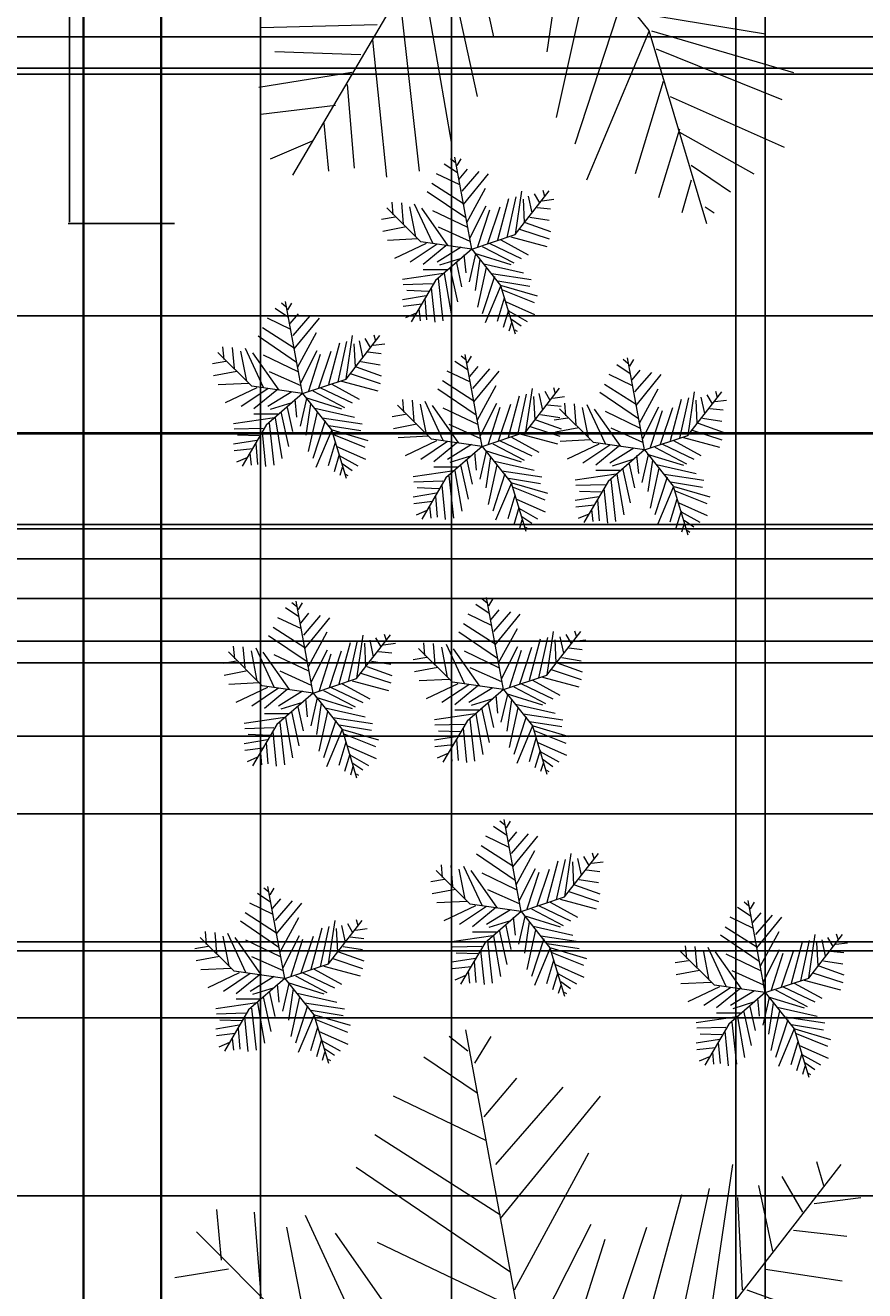
# Model space of a CAD drawing. Units: inches. Extents: x 818 to 1898, y 976 to 2364.
# Tile 6 of 96: x 986 to 1083, y 1446 to 1592. Entities that reach past the tile are written whole.
import ezdxf

# ---------------------------------------------------------------- set-up
doc = ezdxf.new("R2010")
doc.units = ezdxf.units.IN
doc.header["$LTSCALE"] = 5
doc.header["$MEASUREMENT"] = 0
for name, color, linetype, lineweight in [('A-ANNO-DIMS', 2, 'Continuous', 18), ('C-PROP', 7, 'Continuous', 35), ('L-PLNT-BEDS', 94, 'Continuous', 18)]:
    doc.layers.add(name, color=color, linetype=linetype, lineweight=lineweight)
doc.layers.add('L-PLNT', color=116, linetype='Continuous', lineweight=13, true_color=0x136734)
doc.styles.get("Standard").update_dxf_attribs({"font": 'arial.ttf'})
doc.dimstyles.get("Standard").update_dxf_attribs({"dimtxt": 0.18, "dimasz": 0.18, "dimexe": 0.18, "dimexo": 0.0625, "dimgap": 0.09, "dimtad": 0, "dimtih": 1, "dimtoh": 1, "dimdec": 4, "dimzin": 0, "dimdsep": 46, "dimtxsty": 'Standard', "dimcen": 0.09, "dimadec": 0, "dimazin": 0, "dimtfac": 1, "dimtdec": 4, "dimtofl": 0, "dimtmove": 0, "dimatfit": 3, "dimfxl": 1, "dimtolj": 1, "dimtzin": 0, "dimarcsym": 0})

# ---------------------------------------------------------------- blocks, each defined once
blk = doc.blocks.new('SHRUB-ACCENT')
for p, q in [((8.8, 18.63), (7.25, 19.67)), ((8.53, 19.84), (7.99, 20.28)), ((10.44, 9.82), (8.47, 20.47)), ((8.74, 19.5), (9.21, 20.28)), ((9.01, 17.93), (9.96, 19.06)), ((9.08, 17.24), (6.37, 18.54)), ((9.35, 16.54), (11.31, 18.8)), ((9.48, 14.98), (12.39, 18.54)), ((9.75, 13.42), (5.28, 16.46)), ((9.48, 15.07), (5.82, 17.41)), ((9.89, 12.9), (12.06, 16.89)), ((15.49, 11.5), (19.41, 16.55)), ((15.51, 11.51), (16.25, 16.54)), ((17.68, 16.2), (18.29, 15.16)), ((18.69, 16.63), (18.9, 15.94)), ((1.35, 13.77), (1.22, 15.24)), ((2.3, 15.16), (2.51, 12.72)), ((3.25, 14.72), (3.93, 11.25)), ((3.79, 15.07), (5.89, 10.55)), ((10.23, 11.07), (12.12, 14.81)), ((12.33, 10.47), (13.75, 14.72)), ((13.48, 10.9), (14.76, 15.68)), ((14.56, 11.16), (15.58, 15.85)), ((16.39, 15.59), (16.53, 12.9)), ((17, 15.94), (17.41, 14.03)), ((18.62, 15.42), (19.98, 15.59)), ((1.56, 13.51), (0, 13.25)), ((4.55, 10.66), (0.62, 14.58)), ((7.72, 10.21), (4.67, 14.55)), ((5.89, 14.29), (9.89, 12.38)), ((11.17, 10.12), (12.53, 14.37)), ((17.2, 13.51), (19.44, 13.16)), ((18.02, 14.63), (19.57, 14.46)), ((2.84, 12.38), (0.14, 11.86)), ((6.57, 12.38), (10.23, 10.73)), ((15.98, 12.12), (19.44, 10.99)), ((16.66, 12.9), (19.57, 11.86)), ((4.2, 10.99), (0.68, 10.81)), ((5.15, 10.47), (1.49, 8.73)), ((6.43, 10.38), (3.32, 8.3)), ((10.44, 9.82), (4.55, 10.66)), ((10.44, 9.82), (15.49, 11.5)), ((12.53, 10.47), (16.19, 8.73)), ((13.82, 10.9), (17, 9.16)), ((14.97, 11.25), (19.17, 10.12)), ((7.45, 10.21), (4.81, 8.04)), ((10.44, 9.82), (6.23, 6.17)), ((9.21, 10.03), (6.43, 8.3)), ((9.55, 9.16), (9.75, 7.08)), ((10.9, 9.25), (10.16, 6.04)), ((10.44, 9.82), (13.8, 5.61)), ((10.77, 9.34), (14.97, 8.04)), ((11.65, 10.12), (15.31, 8.21)), ((7.59, 7.43), (4.81, 7.43)), ((9.21, 8.73), (6.7, 7.95)), ((7.92, 7.69), (8.8, 3.69)), ((8.67, 8.21), (9.28, 5.43)), ((11.38, 8.64), (10.84, 5)), ((12.12, 7.69), (11.11, 3.09)), ((11.85, 8.12), (16.46, 7.08)), ((7.18, 6.99), (2.44, 6.3)), ((6.23, 6.17), (3.43, 1.4)), ((6.57, 6.39), (7.11, 1.52)), ((7.25, 6.99), (8.06, 2.31)), ((13.07, 6.65), (11.65, 2.31)), ((12.73, 6.99), (17.34, 6.3)), ((13.48, 6.13), (17.2, 5.52)), ((5.89, 5.78), (2.51, 5.69)), ((5.42, 4.91), (2.91, 5)), ((5.76, 5.34), (6.16, 1.35)), ((13.82, 5.6), (11.99, 1.26)), ((13.8, 5.61), (15.49, 0)), ((13.88, 5.6), (18.02, 4.39)), ((14.02, 5.08), (17.68, 3.61)), ((5.15, 4.39), (2.44, 3.95)), ((4.67, 3.43), (2.51, 3.17)), ((5.01, 4.04), (5.21, 1.61)), ((14.22, 4.13), (13.41, 1.44)), ((14.43, 3.69), (17.74, 2.22)), ((4, 2.39), (2.78, 1.87)), ((4.33, 2.91), (4.47, 1.52)), ((14.7, 2.74), (14.09, 0.74)), ((14.7, 2.65), (16.86, 1.44)), ((15.04, 1.7), (16.19, 0.92)), ((15.04, 1.26), (14.76, 0.31)), ((15.44, 0.48), (15.71, 0.31))]:
    blk.add_line(p, q)
blk = doc.blocks.new('PALM-BORDER')
for p, q in [((33.95, 78.95), (31.8, 80.68)), ((41.53, 39.05), (33.72, 81.45)), ((34.76, 77.57), (36.65, 80.68)), ((35.03, 74.11), (28.83, 78.26)), ((35.84, 71.35), (39.61, 75.84)), ((37.18, 65.82), (45, 74.8)), ((36.11, 68.59), (25.33, 73.77)), ((37.72, 59.6), (49.31, 73.77)), ((37.72, 59.95), (23.17, 69.28)), ((39.34, 51.31), (47.96, 67.2)), ((74.37, 66.17), (75.18, 63.4)), ((38.8, 53.39), (21.02, 65.48)), ((61.61, 45.75), (77.23, 65.83)), ((61.71, 45.79), (64.67, 65.82)), ((57.93, 44.41), (61.97, 63.06)), ((67.63, 63.4), (69.25, 55.81)), ((70.33, 64.44), (72.75, 60.3)), ((53.62, 43.37), (58.74, 62.37)), ((65.21, 62.02), (65.75, 51.31)), ((74.1, 61.33), (79.49, 62.02)), ((5.39, 54.77), (4.85, 60.64)), ((9.16, 60.3), (9.97, 50.62)), ((15.09, 59.95), (23.44, 41.99)), ((40.69, 44.06), (48.23, 58.91)), ((18.1, 42.4), (2.48, 58.02)), ((12.93, 58.57), (15.63, 44.75)), ((30.72, 40.61), (18.59, 57.88)), ((44.46, 40.26), (49.85, 57.19)), ((49.04, 41.64), (54.7, 58.57)), ((71.68, 58.22), (77.87, 57.53)), ((23.44, 56.84), (39.34, 49.24)), ((6.2, 53.73), (0, 52.7)), ((68.44, 53.73), (77.33, 52.35)), ((66.29, 51.31), (77.87, 47.17)), ((11.32, 49.24), (0.54, 47.17)), ((26.14, 49.24), (40.69, 42.68)), ((63.59, 48.21), (77.33, 43.71)), ((41.53, 39.05), (61.61, 45.75)), ((59.55, 44.75), (76.26, 40.26)), ((16.71, 43.71), (2.69, 43.02)), ((54.97, 43.37), (67.63, 36.46)), ((20.48, 41.64), (5.93, 34.73)), ((25.6, 41.3), (13.2, 33.01)), ((41.53, 39.05), (18.1, 42.4)), ((49.85, 41.64), (64.4, 34.73)), ((29.64, 40.61), (19.13, 31.97)), ((36.65, 39.91), (25.6, 33.01)), ((46.35, 40.26), (60.9, 32.66)), ((41.53, 39.05), (24.79, 24.55)), ((41.53, 39.05), (54.92, 22.32)), ((43.38, 36.81), (40.42, 24.02)), ((42.84, 37.15), (59.55, 31.97)), ((37.99, 36.46), (38.8, 28.17)), ((36.65, 34.73), (26.68, 31.62)), ((45.27, 34.39), (43.11, 19.88)), ((34.49, 32.66), (36.92, 21.61)), ((47.15, 32.32), (65.48, 28.17)), ((30.18, 29.55), (19.13, 29.55)), ((31.53, 30.59), (35.03, 14.7)), ((48.23, 30.59), (44.19, 12.28)), ((28.56, 27.82), (9.7, 25.06)), ((28.83, 27.82), (32.07, 9.17)), ((52, 26.44), (46.35, 9.17)), ((50.66, 27.82), (68.98, 25.06)), ((26.14, 25.41), (28.29, 6.06)), ((24.79, 24.55), (13.63, 5.58)), ((53.62, 24.37), (68.44, 21.95)), ((23.44, 22.99), (9.97, 22.64)), ((54.97, 22.3), (47.69, 5.02)), ((54.92, 22.32), (61.61, 0)), ((55.24, 22.3), (71.68, 17.46)), ((22.9, 21.26), (24.52, 5.37)), ((21.56, 19.53), (11.59, 19.88)), ((55.78, 20.22), (70.33, 14.35)), ((20.48, 17.46), (9.7, 15.73)), ((56.59, 16.42), (53.35, 5.72)), ((19.94, 16.08), (20.75, 6.41)), ((57.39, 14.7), (70.6, 8.83)), ((18.59, 13.66), (9.97, 12.62)), ((17.24, 11.59), (17.78, 6.06)), ((58.47, 10.9), (56.05, 2.95)), ((58.47, 10.55), (67.09, 5.72)), ((15.9, 9.52), (11.05, 7.44)), ((59.82, 6.75), (64.4, 3.64)), ((59.82, 5.02), (58.74, 1.22)), ((61.44, 1.92), (62.51, 1.22))]:
    blk.add_line(p, q)
blk = doc.blocks.new('*D26')
at = {"layer": 'A-ANNO-DIMS', "color": 0, "lineweight": -2, "ltscale": 5, "transparency": 16777216}
for p, q in [((1003.26, 1650.91), (990.92, 1650.91)), ((991.1, 1650.73), (991.1, 1610.37)), ((991.1, 1569.64), (991.1, 1610)), ((1003.26, 1569.46), (990.92, 1569.46))]:
    blk.add_line(p, q, dxfattribs=at)
at = {"layer": 'A-ANNO-DIMS', "color": 0, "ltscale": 5, "transparency": 16777216}
for points in [[(991.07, 1650.73), (991.13, 1650.73), (991.1, 1650.91)], [(991.07, 1569.64), (991.13, 1569.64), (991.1, 1569.46)]]:
    blk.add_solid(points, dxfattribs=at)
at = {"layer": 'Defpoints', "color": 0, "ltscale": 5, "transparency": 16777216}
for p in [(991.1, 1650.91), (1003.32, 1650.91), (1003.32, 1569.46)]:
    blk.add_point(p, dxfattribs=at)
at = {"layer": 'A-ANNO-DIMS', "color": 0, "ltscale": 5, "transparency": 16777216, "insert": (991.1, 1610.19), "char_height": 0.18, "attachment_point": 5}
blk.add_mtext('\\A1;BORDER PALM 81 TYP.', dxfattribs=at)
blk = doc.blocks.new('*D59')
at = {"layer": 'A-ANNO-DIMS', "color": 0, "lineweight": -2, "ltscale": 5, "transparency": 16777216}
for p, q in [((1251.64, 2300.39), (818.03, 2300.39)), ((818.21, 2300.21), (818.21, 1669.95)), ((818.21, 1039.32), (818.21, 1669.59)), ((896.05, 1039.14), (818.03, 1039.14))]:
    blk.add_line(p, q, dxfattribs=at)
at = {"layer": 'A-ANNO-DIMS', "color": 0, "ltscale": 5, "transparency": 16777216}
for points in [[(818.18, 2300.21), (818.24, 2300.21), (818.21, 2300.39)], [(818.18, 1039.32), (818.24, 1039.32), (818.21, 1039.14)]]:
    blk.add_solid(points, dxfattribs=at)
at = {"layer": 'Defpoints', "color": 0, "ltscale": 5, "transparency": 16777216}
for p in [(818.21, 2300.39), (1251.71, 2300.39), (896.11, 1039.14)]:
    blk.add_point(p, dxfattribs=at)
at = {"layer": 'A-ANNO-DIMS', "color": 0, "ltscale": 5, "transparency": 16777216, "insert": (818.21, 1669.77), "char_height": 0.18, "attachment_point": 5}
blk.add_mtext('\\A1;1261.2', dxfattribs=at)
blk = doc.blocks.new('*D60')
at = {"layer": 'A-ANNO-DIMS', "color": 0, "lineweight": -2, "ltscale": 5, "transparency": 16777216}
for p, q in [((992.66, 2294.22), (818.03, 2294.22)), ((818.21, 2294.04), (818.21, 1748.77)), ((818.21, 1203.14), (818.21, 1748.41)), ((992.66, 1202.96), (818.03, 1202.96))]:
    blk.add_line(p, q, dxfattribs=at)
at = {"layer": 'A-ANNO-DIMS', "color": 0, "ltscale": 5, "transparency": 16777216}
for points in [[(818.18, 2294.04), (818.24, 2294.04), (818.21, 2294.22)], [(818.18, 1203.14), (818.24, 1203.14), (818.21, 1202.96)]]:
    blk.add_solid(points, dxfattribs=at)
at = {"layer": 'Defpoints', "color": 0, "ltscale": 5, "transparency": 16777216}
for p in [(818.21, 2294.22), (992.73, 2294.22), (992.73, 1202.96)]:
    blk.add_point(p, dxfattribs=at)
at = {"layer": 'A-ANNO-DIMS', "color": 0, "ltscale": 5, "transparency": 16777216, "insert": (818.21, 1748.59), "char_height": 0.18, "attachment_point": 5}
blk.add_mtext('\\A1;1091.3', dxfattribs=at)
blk = doc.blocks.new('*D61')
at = {"layer": 'A-ANNO-DIMS', "color": 0, "lineweight": -2, "ltscale": 5, "transparency": 16777216}
for p, q in [((1071.73, 1203.03), (1071.73, 2363.87)), ((1071.91, 2363.69), (1250.94, 2363.69)), ((1430.55, 2363.69), (1251.51, 2363.69)), ((1430.73, 1203.03), (1430.73, 2363.87))]:
    blk.add_line(p, q, dxfattribs=at)
at = {"layer": 'A-ANNO-DIMS', "color": 0, "ltscale": 5, "transparency": 16777216}
for points in [[(1071.91, 2363.72), (1071.91, 2363.66), (1071.73, 2363.69)], [(1430.55, 2363.72), (1430.55, 2363.66), (1430.73, 2363.69)]]:
    blk.add_solid(points, dxfattribs=at)
at = {"layer": 'Defpoints', "color": 0, "ltscale": 5, "transparency": 16777216}
for p in [(1430.73, 2363.69), (1071.73, 1202.96), (1430.73, 1202.96)]:
    blk.add_point(p, dxfattribs=at)
at = {"layer": 'A-ANNO-DIMS', "color": 0, "ltscale": 5, "transparency": 16777216, "insert": (1251.23, 2363.69), "char_height": 0.18, "attachment_point": 5}
blk.add_mtext('\\A1;359', dxfattribs=at)
blk = doc.blocks.new('*D63')
at = {"layer": 'A-ANNO-DIMS', "color": 0, "lineweight": -2, "ltscale": 5, "transparency": 16777216}
for p, q in [((1116.13, 1485.2), (818.03, 1485.2)), ((818.21, 1485.02), (818.21, 1360.77)), ((818.21, 1236.14), (818.21, 1360.4)), ((1116.13, 1235.96), (818.03, 1235.96))]:
    blk.add_line(p, q, dxfattribs=at)
at = {"layer": 'A-ANNO-DIMS', "color": 0, "ltscale": 5, "transparency": 16777216}
for points in [[(818.18, 1485.02), (818.24, 1485.02), (818.21, 1485.2)], [(818.18, 1236.14), (818.24, 1236.14), (818.21, 1235.96)]]:
    blk.add_solid(points, dxfattribs=at)
at = {"layer": 'Defpoints', "color": 0, "ltscale": 5, "transparency": 16777216}
for p in [(818.21, 1485.2), (1116.19, 1485.2), (1116.19, 1235.96)]:
    blk.add_point(p, dxfattribs=at)
at = {"layer": 'A-ANNO-DIMS', "color": 0, "ltscale": 5, "transparency": 16777216, "insert": (818.21, 1360.58), "char_height": 0.18, "attachment_point": 5}
blk.add_mtext('\\A1;249.24', dxfattribs=at)
blk = doc.blocks.new('*D79')
at = {"layer": 'A-ANNO-DIMS', "color": 0, "lineweight": -2, "ltscale": 5, "transparency": 16777216}
for p, q in [((992.73, 1203.03), (992.73, 2363.87)), ((992.91, 2363.69), (1032.01, 2363.69)), ((1071.55, 2363.69), (1032.44, 2363.69)), ((1071.73, 1203.03), (1071.73, 2363.87))]:
    blk.add_line(p, q, dxfattribs=at)
at = {"layer": 'A-ANNO-DIMS', "color": 0, "ltscale": 5, "transparency": 16777216}
for points in [[(992.91, 2363.72), (992.91, 2363.66), (992.73, 2363.69)], [(1071.55, 2363.72), (1071.55, 2363.66), (1071.73, 2363.69)]]:
    blk.add_solid(points, dxfattribs=at)
at = {"layer": 'Defpoints', "color": 0, "ltscale": 5, "transparency": 16777216}
for p in [(1071.73, 2363.69), (992.73, 1202.96), (1071.73, 1202.96)]:
    blk.add_point(p, dxfattribs=at)
at = {"layer": 'A-ANNO-DIMS', "color": 0, "ltscale": 5, "transparency": 16777216, "insert": (1032.23, 2363.69), "char_height": 0.18, "attachment_point": 5}
blk.add_mtext('\\A1;79', dxfattribs=at)
blk = doc.blocks.new('*D84')
at = {"layer": 'A-ANNO-DIMS', "color": 0, "lineweight": -2, "ltscale": 5, "transparency": 16777216}
for p, q in [((1197.66, 1700.08), (818.03, 1700.08)), ((818.21, 1699.9), (818.21, 1600.76)), ((818.21, 1501.26), (818.21, 1600.4)), ((1197.66, 1501.08), (818.03, 1501.08))]:
    blk.add_line(p, q, dxfattribs=at)
at = {"layer": 'A-ANNO-DIMS', "color": 0, "ltscale": 5, "transparency": 16777216}
for points in [[(818.18, 1699.9), (818.24, 1699.9), (818.21, 1700.08)], [(818.18, 1501.26), (818.24, 1501.26), (818.21, 1501.08)]]:
    blk.add_solid(points, dxfattribs=at)
at = {"layer": 'Defpoints', "color": 0, "ltscale": 5, "transparency": 16777216}
for p in [(818.21, 1700.08), (1197.73, 1700.08), (1197.73, 1501.08)]:
    blk.add_point(p, dxfattribs=at)
at = {"layer": 'A-ANNO-DIMS', "color": 0, "ltscale": 5, "transparency": 16777216, "insert": (818.21, 1600.58), "char_height": 0.18, "attachment_point": 5}
blk.add_mtext('\\A1;199', dxfattribs=at)
blk = doc.blocks.new('*D91')
at = {"layer": 'A-ANNO-DIMS', "color": 0, "lineweight": -2, "ltscale": 5, "transparency": 16777216}
for p, q in [((959.17, 1071.12), (959.17, 2363.87)), ((959.35, 2363.69), (985.8, 2363.69)), ((1013.04, 2363.69), (986.59, 2363.69)), ((1013.22, 1071.12), (1013.22, 2363.87))]:
    blk.add_line(p, q, dxfattribs=at)
at = {"layer": 'A-ANNO-DIMS', "color": 0, "ltscale": 5, "transparency": 16777216}
for points in [[(959.35, 2363.72), (959.35, 2363.66), (959.17, 2363.69)], [(1013.04, 2363.72), (1013.04, 2363.66), (1013.22, 2363.69)]]:
    blk.add_solid(points, dxfattribs=at)
at = {"layer": 'Defpoints', "color": 0, "ltscale": 5, "transparency": 16777216}
for p in [(1013.22, 2363.69), (959.17, 1071.06), (1013.22, 1071.06)]:
    blk.add_point(p, dxfattribs=at)
at = {"layer": 'A-ANNO-DIMS', "color": 0, "ltscale": 5, "transparency": 16777216, "insert": (986.2, 2363.69), "char_height": 0.18, "attachment_point": 5}
blk.add_mtext('\\A1;54.04', dxfattribs=at)
blk = doc.blocks.new('*D92')
at = {"layer": 'A-ANNO-DIMS', "color": 0, "lineweight": -2, "ltscale": 5, "transparency": 16777216}
for p, q in [((1013.22, 1071.12), (1013.22, 2363.87)), ((1013.4, 2363.69), (1040.38, 2363.69)), ((1068.16, 2363.69), (1041.17, 2363.69)), ((1068.34, 1071.12), (1068.34, 2363.87))]:
    blk.add_line(p, q, dxfattribs=at)
at = {"layer": 'A-ANNO-DIMS', "color": 0, "ltscale": 5, "transparency": 16777216}
for points in [[(1013.4, 2363.72), (1013.4, 2363.66), (1013.22, 2363.69)], [(1068.16, 2363.72), (1068.16, 2363.66), (1068.34, 2363.69)]]:
    blk.add_solid(points, dxfattribs=at)
at = {"layer": 'Defpoints', "color": 0, "ltscale": 5, "transparency": 16777216}
for p in [(1068.34, 2363.69), (1013.22, 1071.06), (1068.34, 1071.06)]:
    blk.add_point(p, dxfattribs=at)
at = {"layer": 'A-ANNO-DIMS', "color": 0, "ltscale": 5, "transparency": 16777216, "insert": (1040.78, 2363.69), "char_height": 0.18, "attachment_point": 5}
blk.add_mtext('\\A1;55.12', dxfattribs=at)
blk = doc.blocks.new('*D93')
at = {"layer": 'A-ANNO-DIMS', "color": 0, "lineweight": -2, "ltscale": 5, "transparency": 16777216}
for p, q in [((1068.34, 1071.12), (1068.34, 2363.87)), ((1068.52, 2363.69), (1094.16, 2363.69)), ((1120.58, 2363.69), (1094.94, 2363.69)), ((1120.76, 1071.12), (1120.76, 2363.87))]:
    blk.add_line(p, q, dxfattribs=at)
at = {"layer": 'A-ANNO-DIMS', "color": 0, "ltscale": 5, "transparency": 16777216}
for points in [[(1068.52, 2363.72), (1068.52, 2363.66), (1068.34, 2363.69)], [(1120.58, 2363.72), (1120.58, 2363.66), (1120.76, 2363.69)]]:
    blk.add_solid(points, dxfattribs=at)
at = {"layer": 'Defpoints', "color": 0, "ltscale": 5, "transparency": 16777216}
for p in [(1120.76, 2363.69), (1068.34, 1071.06), (1120.76, 1071.06)]:
    blk.add_point(p, dxfattribs=at)
at = {"layer": 'A-ANNO-DIMS', "color": 0, "ltscale": 5, "transparency": 16777216, "insert": (1094.55, 2363.69), "char_height": 0.18, "attachment_point": 5}
blk.add_mtext('\\A1;52.42', dxfattribs=at)
blk = doc.blocks.new('*D116')
at = {"layer": 'A-ANNO-DIMS', "color": 0, "lineweight": -2, "ltscale": 5, "transparency": 16777216}
for p, q in [((1766.29, 1456.81), (818.03, 1456.81)), ((818.21, 1456.63), (818.21, 1417.41)), ((818.21, 1377.84), (818.21, 1417.05)), ((1766.29, 1377.66), (818.03, 1377.66))]:
    blk.add_line(p, q, dxfattribs=at)
at = {"layer": 'A-ANNO-DIMS', "color": 0, "ltscale": 5, "transparency": 16777216}
for points in [[(818.18, 1456.63), (818.24, 1456.63), (818.21, 1456.81)], [(818.18, 1377.84), (818.24, 1377.84), (818.21, 1377.66)]]:
    blk.add_solid(points, dxfattribs=at)
at = {"layer": 'Defpoints', "color": 0, "ltscale": 5, "transparency": 16777216}
for p in [(818.21, 1456.81), (1766.35, 1456.81), (1766.35, 1377.66)]:
    blk.add_point(p, dxfattribs=at)
at = {"layer": 'A-ANNO-DIMS', "color": 0, "ltscale": 5, "transparency": 16777216, "insert": (818.21, 1417.23), "char_height": 0.18, "attachment_point": 5}
blk.add_mtext('\\A1;79.15', dxfattribs=at)
blk = doc.blocks.new('*D117')
at = {"layer": 'A-ANNO-DIMS', "color": 0, "lineweight": -2, "ltscale": 5, "transparency": 16777216}
for p, q in [((1766.29, 1545.18), (818.03, 1545.18)), ((818.21, 1545), (818.21, 1501.18)), ((818.21, 1456.99), (818.21, 1500.81)), ((1766.29, 1456.81), (818.03, 1456.81))]:
    blk.add_line(p, q, dxfattribs=at)
at = {"layer": 'A-ANNO-DIMS', "color": 0, "ltscale": 5, "transparency": 16777216}
for points in [[(818.18, 1545), (818.24, 1545), (818.21, 1545.18)], [(818.18, 1456.99), (818.24, 1456.99), (818.21, 1456.81)]]:
    blk.add_solid(points, dxfattribs=at)
at = {"layer": 'Defpoints', "color": 0, "ltscale": 5, "transparency": 16777216}
for p in [(818.21, 1545.18), (1766.35, 1545.18), (1766.35, 1456.81)]:
    blk.add_point(p, dxfattribs=at)
at = {"layer": 'A-ANNO-DIMS', "color": 0, "ltscale": 5, "transparency": 16777216, "insert": (818.21, 1501), "char_height": 0.18, "attachment_point": 5}
blk.add_mtext('\\A1;88.37', dxfattribs=at)
blk = doc.blocks.new('*D118')
at = {"layer": 'A-ANNO-DIMS', "color": 0, "lineweight": -2, "ltscale": 5, "transparency": 16777216}
for p, q in [((1766.29, 1627.51), (818.03, 1627.51)), ((818.21, 1627.33), (818.21, 1586.53)), ((818.21, 1545.36), (818.21, 1586.16)), ((1766.29, 1545.18), (818.03, 1545.18))]:
    blk.add_line(p, q, dxfattribs=at)
at = {"layer": 'A-ANNO-DIMS', "color": 0, "ltscale": 5, "transparency": 16777216}
for points in [[(818.18, 1627.33), (818.24, 1627.33), (818.21, 1627.51)], [(818.18, 1545.36), (818.24, 1545.36), (818.21, 1545.18)]]:
    blk.add_solid(points, dxfattribs=at)
at = {"layer": 'Defpoints', "color": 0, "ltscale": 5, "transparency": 16777216}
for p in [(818.21, 1627.51), (1766.35, 1627.51), (1766.35, 1545.18)]:
    blk.add_point(p, dxfattribs=at)
at = {"layer": 'A-ANNO-DIMS', "color": 0, "ltscale": 5, "transparency": 16777216, "insert": (818.21, 1586.34), "char_height": 0.18, "attachment_point": 5}
blk.add_mtext('\\A1;82.32', dxfattribs=at)
blk = doc.blocks.new('*D122')
at = {"layer": 'A-ANNO-DIMS', "color": 0, "lineweight": -2, "ltscale": 5, "transparency": 16777216}
for p, q in [((1138.5, 1794.37), (1138.5, 975.66)), ((1071.73, 1688.02), (1071.73, 975.66)), ((1071.91, 975.84), (1104.72, 975.84)), ((1138.32, 975.84), (1105.51, 975.84))]:
    blk.add_line(p, q, dxfattribs=at)
at = {"layer": 'A-ANNO-DIMS', "color": 0, "ltscale": 5, "transparency": 16777216}
for points in [[(1071.91, 975.87), (1071.91, 975.81), (1071.73, 975.84)], [(1138.32, 975.87), (1138.32, 975.81), (1138.5, 975.84)]]:
    blk.add_solid(points, dxfattribs=at)
at = {"layer": 'Defpoints', "color": 0, "ltscale": 5, "transparency": 16777216}
for p in [(1138.5, 1794.43), (1071.73, 1688.08), (1138.5, 975.84)]:
    blk.add_point(p, dxfattribs=at)
at = {"layer": 'A-ANNO-DIMS', "color": 0, "ltscale": 5, "transparency": 16777216, "insert": (1105.11, 975.84), "char_height": 0.18, "attachment_point": 5}
blk.add_mtext('\\A1;66.78', dxfattribs=at)
blk = doc.blocks.new('*D126')
at = {"layer": 'A-ANNO-DIMS', "color": 0, "lineweight": -2, "ltscale": 5, "transparency": 16777216}
for p, q in [((1035.38, 1252.09), (1035.38, 2363.87)), ((1035.56, 2363.69), (1075.41, 2363.69)), ((1116.01, 2363.69), (1076.16, 2363.69)), ((1116.19, 1236.03), (1116.19, 2363.87))]:
    blk.add_line(p, q, dxfattribs=at)
at = {"layer": 'A-ANNO-DIMS', "color": 0, "ltscale": 5, "transparency": 16777216}
for points in [[(1035.56, 2363.72), (1035.56, 2363.66), (1035.38, 2363.69)], [(1116.01, 2363.72), (1116.01, 2363.66), (1116.19, 2363.69)]]:
    blk.add_solid(points, dxfattribs=at)
at = {"layer": 'Defpoints', "color": 0, "ltscale": 5, "transparency": 16777216}
for p in [(1035.38, 2363.69), (1035.38, 1252.02), (1116.19, 1235.96)]:
    blk.add_point(p, dxfattribs=at)
at = {"layer": 'A-ANNO-DIMS', "color": 0, "ltscale": 5, "transparency": 16777216, "insert": (1075.78, 2363.69), "char_height": 0.18, "attachment_point": 5}
blk.add_mtext('\\A1;80.81', dxfattribs=at)
blk = doc.blocks.new('*D129')
at = {"layer": 'A-ANNO-DIMS', "color": 0, "lineweight": -2, "ltscale": 5, "transparency": 16777216}
for p, q in [((1044.78, 1608.51), (818.03, 1608.51)), ((818.21, 1608.33), (818.21, 1521.27)), ((818.21, 1433.85), (818.21, 1520.91)), ((1044.78, 1433.67), (818.03, 1433.67))]:
    blk.add_line(p, q, dxfattribs=at)
at = {"layer": 'A-ANNO-DIMS', "color": 0, "ltscale": 5, "transparency": 16777216}
for points in [[(818.18, 1608.33), (818.24, 1608.33), (818.21, 1608.51)], [(818.18, 1433.85), (818.24, 1433.85), (818.21, 1433.67)]]:
    blk.add_solid(points, dxfattribs=at)
at = {"layer": 'Defpoints', "color": 0, "ltscale": 5, "transparency": 16777216}
for p in [(818.21, 1608.51), (1044.85, 1608.51), (1044.85, 1433.67)]:
    blk.add_point(p, dxfattribs=at)
at = {"layer": 'A-ANNO-DIMS', "color": 0, "ltscale": 5, "transparency": 16777216, "insert": (818.21, 1521.09), "char_height": 0.18, "attachment_point": 5}
blk.add_mtext('\\A1;174.84', dxfattribs=at)
blk = doc.blocks.new('*D156')
at = {"layer": 'A-ANNO-DIMS', "color": 0, "lineweight": -2, "ltscale": 5, "transparency": 16777216}
for p, q in [((1177.66, 1586.76), (818.03, 1586.76)), ((818.21, 1586.58), (818.21, 1560.86)), ((818.21, 1534.78), (818.21, 1560.5)), ((1177.66, 1534.6), (818.03, 1534.6))]:
    blk.add_line(p, q, dxfattribs=at)
at = {"layer": 'A-ANNO-DIMS', "color": 0, "ltscale": 5, "transparency": 16777216}
for points in [[(818.18, 1586.58), (818.24, 1586.58), (818.21, 1586.76)], [(818.18, 1534.78), (818.24, 1534.78), (818.21, 1534.6)]]:
    blk.add_solid(points, dxfattribs=at)
at = {"layer": 'Defpoints', "color": 0, "ltscale": 5, "transparency": 16777216}
for p in [(818.21, 1586.76), (1177.73, 1586.76), (1177.73, 1534.6)]:
    blk.add_point(p, dxfattribs=at)
at = {"layer": 'A-ANNO-DIMS', "color": 0, "ltscale": 5, "transparency": 16777216, "insert": (818.21, 1560.68), "char_height": 0.18, "attachment_point": 5}
blk.add_mtext('\\A1;52.16', dxfattribs=at)
blk = doc.blocks.new('*D157')
at = {"layer": 'A-ANNO-DIMS', "color": 0, "lineweight": -2, "ltscale": 5, "transparency": 16777216}
for p, q in [((1197.66, 1530.6), (818.03, 1530.6)), ((818.21, 1530.42), (818.21, 1516.02)), ((818.21, 1501.26), (818.21, 1515.66)), ((1197.66, 1501.08), (818.03, 1501.08))]:
    blk.add_line(p, q, dxfattribs=at)
at = {"layer": 'A-ANNO-DIMS', "color": 0, "ltscale": 5, "transparency": 16777216}
for points in [[(818.18, 1530.42), (818.24, 1530.42), (818.21, 1530.6)], [(818.18, 1501.26), (818.24, 1501.26), (818.21, 1501.08)]]:
    blk.add_solid(points, dxfattribs=at)
at = {"layer": 'Defpoints', "color": 0, "ltscale": 5, "transparency": 16777216}
for p in [(818.21, 1530.6), (1197.73, 1530.6), (1197.73, 1501.08)]:
    blk.add_point(p, dxfattribs=at)
at = {"layer": 'A-ANNO-DIMS', "color": 0, "ltscale": 5, "transparency": 16777216, "insert": (818.21, 1515.84), "char_height": 0.18, "attachment_point": 5}
blk.add_mtext('\\A1;29.524', dxfattribs=at)
blk = doc.blocks.new('*D168')
at = {"layer": 'A-ANNO-DIMS', "color": 0, "lineweight": -2, "ltscale": 5, "transparency": 16777216}
for p, q in [((1430.66, 1501.08), (818.03, 1501.08)), ((818.21, 1500.9), (818.21, 1493.84)), ((818.21, 1486.42), (818.21, 1493.48)), ((1430.66, 1486.24), (818.03, 1486.24))]:
    blk.add_line(p, q, dxfattribs=at)
at = {"layer": 'A-ANNO-DIMS', "color": 0, "ltscale": 5, "transparency": 16777216}
for points in [[(818.18, 1500.9), (818.24, 1500.9), (818.21, 1501.08)], [(818.18, 1486.42), (818.24, 1486.42), (818.21, 1486.24)]]:
    blk.add_solid(points, dxfattribs=at)
at = {"layer": 'Defpoints', "color": 0, "ltscale": 5, "transparency": 16777216}
for p in [(818.21, 1501.08), (1430.73, 1501.08), (1430.73, 1486.24)]:
    blk.add_point(p, dxfattribs=at)
at = {"layer": 'A-ANNO-DIMS', "color": 0, "ltscale": 5, "transparency": 16777216, "insert": (818.21, 1493.66), "char_height": 0.18, "attachment_point": 5}
blk.add_mtext('\\A1;14.84', dxfattribs=at)
blk = doc.blocks.new('*D187')
at = {"layer": 'A-ANNO-DIMS', "color": 0, "lineweight": -2, "ltscale": 5, "transparency": 16777216}
for p, q in [((1705.66, 1545.08), (818.03, 1545.08)), ((818.21, 1544.9), (818.21, 1533.26)), ((818.21, 1521.26), (818.21, 1532.9)), ((1705.66, 1521.08), (818.03, 1521.08))]:
    blk.add_line(p, q, dxfattribs=at)
at = {"layer": 'A-ANNO-DIMS', "color": 0, "ltscale": 5, "transparency": 16777216}
for points in [[(818.18, 1544.9), (818.24, 1544.9), (818.21, 1545.08)], [(818.18, 1521.26), (818.24, 1521.26), (818.21, 1521.08)]]:
    blk.add_solid(points, dxfattribs=at)
at = {"layer": 'Defpoints', "color": 0, "ltscale": 5, "transparency": 16777216}
for p in [(818.21, 1545.08), (1705.73, 1545.08), (1705.73, 1521.08)]:
    blk.add_point(p, dxfattribs=at)
at = {"layer": 'A-ANNO-DIMS', "color": 0, "ltscale": 5, "transparency": 16777216, "insert": (818.21, 1533.08), "char_height": 0.18, "attachment_point": 5}
blk.add_mtext('\\A1;24', dxfattribs=at)
blk = doc.blocks.new('*D194')
at = {"layer": 'A-ANNO-DIMS', "color": 0, "lineweight": -2, "ltscale": 5, "transparency": 16777216}
for p, q in [((1616.66, 1591.08), (818.03, 1591.08)), ((818.21, 1590.9), (818.21, 1575.1)), ((818.21, 1558.93), (818.21, 1574.73)), ((1616.66, 1558.75), (818.03, 1558.75))]:
    blk.add_line(p, q, dxfattribs=at)
at = {"layer": 'A-ANNO-DIMS', "color": 0, "ltscale": 5, "transparency": 16777216}
for points in [[(818.18, 1590.9), (818.24, 1590.9), (818.21, 1591.08)], [(818.18, 1558.93), (818.24, 1558.93), (818.21, 1558.75)]]:
    blk.add_solid(points, dxfattribs=at)
at = {"layer": 'Defpoints', "color": 0, "ltscale": 5, "transparency": 16777216}
for p in [(818.21, 1591.08), (1616.73, 1591.08), (1616.73, 1558.75)]:
    blk.add_point(p, dxfattribs=at)
at = {"layer": 'A-ANNO-DIMS', "color": 0, "ltscale": 5, "transparency": 16777216, "insert": (818.21, 1574.92), "char_height": 0.18, "attachment_point": 5}
blk.add_mtext('\\A1;32.326', dxfattribs=at)
blk = doc.blocks.new('*D201')
at = {"layer": 'A-ANNO-DIMS', "color": 0, "lineweight": -2, "ltscale": 5, "transparency": 16777216}
for p, q in [((1678.27, 1518.56), (818.03, 1518.56)), ((818.21, 1518.38), (818.21, 1498.18)), ((818.21, 1477.61), (818.21, 1497.81)), ((1678.27, 1477.43), (818.03, 1477.43))]:
    blk.add_line(p, q, dxfattribs=at)
at = {"layer": 'A-ANNO-DIMS', "color": 0, "ltscale": 5, "transparency": 16777216}
for points in [[(818.18, 1518.38), (818.24, 1518.38), (818.21, 1518.56)], [(818.18, 1477.61), (818.24, 1477.61), (818.21, 1477.43)]]:
    blk.add_solid(points, dxfattribs=at)
at = {"layer": 'Defpoints', "color": 0, "ltscale": 5, "transparency": 16777216}
for p in [(818.21, 1518.56), (1678.33, 1518.56), (1678.33, 1477.43)]:
    blk.add_point(p, dxfattribs=at)
at = {"layer": 'A-ANNO-DIMS', "color": 0, "ltscale": 5, "transparency": 16777216, "insert": (818.21, 1497.99), "char_height": 0.18, "attachment_point": 5}
blk.add_mtext('\\A1;41.135', dxfattribs=at)
blk = doc.blocks.new('*D270')
at = {"layer": 'A-ANNO-DIMS', "color": 0, "lineweight": -2, "ltscale": 5, "transparency": 16777216}
for p, q in [((1246.88, 1534.08), (818.03, 1534.08)), ((818.21, 1533.9), (818.21, 1522.26)), ((818.21, 1510.26), (818.21, 1521.9)), ((1246.88, 1510.08), (818.03, 1510.08))]:
    blk.add_line(p, q, dxfattribs=at)
at = {"layer": 'A-ANNO-DIMS', "color": 0, "ltscale": 5, "transparency": 16777216}
for points in [[(818.18, 1533.9), (818.24, 1533.9), (818.21, 1534.08)], [(818.18, 1510.26), (818.24, 1510.26), (818.21, 1510.08)]]:
    blk.add_solid(points, dxfattribs=at)
at = {"layer": 'Defpoints', "color": 0, "ltscale": 5, "transparency": 16777216}
for p in [(818.21, 1534.08), (1246.94, 1534.08), (1246.94, 1510.08)]:
    blk.add_point(p, dxfattribs=at)
at = {"layer": 'A-ANNO-DIMS', "color": 0, "ltscale": 5, "transparency": 16777216, "insert": (818.21, 1522.08), "char_height": 0.18, "attachment_point": 5}
blk.add_mtext('\\A1;24', dxfattribs=at)
blk = doc.blocks.new('*D272')
at = {"layer": 'A-ANNO-DIMS', "color": 0, "lineweight": -2, "ltscale": 5, "transparency": 16777216}
for p, q in [((1406.66, 1587.42), (818.03, 1587.42)), ((818.21, 1587.24), (818.21, 1556.89)), ((818.21, 1526.18), (818.21, 1556.52)), ((1406.66, 1526), (818.03, 1526))]:
    blk.add_line(p, q, dxfattribs=at)
at = {"layer": 'A-ANNO-DIMS', "color": 0, "ltscale": 5, "transparency": 16777216}
for points in [[(818.18, 1587.24), (818.24, 1587.24), (818.21, 1587.42)], [(818.18, 1526.18), (818.24, 1526.18), (818.21, 1526)]]:
    blk.add_solid(points, dxfattribs=at)
at = {"layer": 'Defpoints', "color": 0, "ltscale": 5, "transparency": 16777216}
for p in [(818.21, 1587.42), (1406.73, 1587.42), (1406.73, 1526)]:
    blk.add_point(p, dxfattribs=at)
at = {"layer": 'A-ANNO-DIMS', "color": 0, "ltscale": 5, "transparency": 16777216, "insert": (818.21, 1556.71), "char_height": 0.18, "attachment_point": 5}
blk.add_mtext('\\A1;61.42', dxfattribs=at)

msp = doc.modelspace()

# ---------------------------------------------------------------- linework, layer by layer
at = {"layer": 'C-PROP'}
for p, q in [((992.7251, 2294.2171), (992.7251, 1202.9642)), ((1001.7252, 2285.2171), (1001.7252, 1211.9642))]:
    msp.add_line(p, q, dxfattribs=at)
at = {"layer": 'L-PLNT-BEDS'}
msp.add_line((1071.7251, 2214.9709), (1071.7251, 1202.9642), dxfattribs=at)

# ---------------------------------------------------------------- block references
at = {"layer": 'L-PLNT'}
for name, p in [('PALM-BORDER', (1003.3185, 1569.4605)), ('SHRUB-ACCENT', (1027.2679, 1556.6656)), ('SHRUB-ACCENT', (1007.6614, 1539.9321)), ('SHRUB-ACCENT', (1028.4933, 1533.81)), ('SHRUB-ACCENT', (1047.2829, 1533.4019)), ('SHRUB-ACCENT', (1030.9441, 1505.6488)), ('SHRUB-ACCENT', (1008.8868, 1505.2406)), ('SHRUB-ACCENT', (1032.9864, 1479.9363)), ('SHRUB-ACCENT', (1005.619, 1472.1818)), ('SHRUB-ACCENT', (1061.2873, 1470.5492)), ('PALM-BORDER', (1003.3185, 1394.616))]:
    msp.add_blockref(name, p, dxfattribs=at)

# ---------------------------------------------------------------- dimensions: what is measured, and where the dimension line sits
at = {"layer": 'A-ANNO-DIMS', "ltscale": 5}
for base, p1, p2, override, picture, middle in [((1013.2176, 2363.6929), (959.1737, 1071.0552), (1013.2176, 1071.0552), {"dimdec": 2, "dimlfac": 1, "dimrnd": 0, "dimzin": 0, "dimdsep": 46, "dimlunit": 2}, '*D91', (986.1956, 2363.6929)), ((1071.7251, 2363.6929), (992.7251, 1202.9642), (1071.7251, 1202.9642), {"dimdec": 0, "dimlfac": 1, "dimrnd": 0, "dimzin": 0, "dimdsep": 46, "dimlunit": 2}, '*D79', (1032.2251, 2363.6929)), ((1068.3377, 2363.6929), (1013.2176, 1071.0552), (1068.3377, 1071.0552), {"dimdec": 2, "dimlfac": 1, "dimrnd": 0, "dimzin": 0, "dimdsep": 46, "dimlunit": 2}, '*D92', (1040.7776, 2363.6929)), ((1035.3768, 2363.6929), (1116.1882, 1235.9642), (1035.3768, 1252.0242), {"dimdec": 2, "dimlfac": 1, "dimrnd": 0, "dimzin": 0, "dimdsep": 46, "dimlunit": 2}, '*D126', (1075.7825, 2363.6929)), ((1120.7618, 2363.6929), (1068.3377, 1071.0552), (1120.7618, 1071.0552), {"dimdec": 2, "dimlfac": 1, "dimrnd": 0, "dimzin": 0, "dimdsep": 46, "dimlunit": 2}, '*D93', (1094.5497, 2363.6929)), ((1430.7251, 2363.6929), (1071.7251, 1202.9642), (1430.7251, 1202.9642), {"dimdec": 0, "dimlfac": 1, "dimrnd": 0, "dimzin": 0, "dimdsep": 46, "dimlunit": 2}, '*D61', (1251.2251, 2363.6929)), ((1138.5041, 975.8433), (1071.7251, 1688.0782), (1138.5041, 1794.4325), {"dimdec": 2, "dimlfac": 1, "dimrnd": 0, "dimzin": 0, "dimdsep": 46, "dimlunit": 2}, '*D122', (1105.1146, 975.8433))]:
    dim = msp.add_linear_dim(base=base, p1=p1, p2=p2, dimstyle='Standard', override=override, dxfattribs=at)
    dim.commit()
    dim.dimension.update_dxf_attribs({"geometry": picture, "text_midpoint": middle})
for base, p1, p2, override, picture, middle in [((818.2059, 2300.3929), (896.1138, 1039.1433), (1251.7057, 2300.3929), {"dimdec": 1, "dimlfac": 1, "dimrnd": 0, "dimzin": 0, "dimdsep": 46, "dimlunit": 2}, '*D59', (818.2059, 1669.7681)), ((818.2059, 2294.2171), (992.7251, 1202.9642), (992.7251, 2294.2171), {"dimdec": 1, "dimlfac": 1, "dimrnd": 0, "dimzin": 0, "dimdsep": 46, "dimlunit": 2}, '*D60', (818.2059, 1748.5907)), ((818.2059, 1700.0782), (1197.7251, 1501.0782), (1197.7251, 1700.0782), {"dimdec": 0, "dimlfac": 1, "dimrnd": 0, "dimzin": 0, "dimdsep": 46, "dimlunit": 2}, '*D84', (818.2059, 1600.5782)), ((818.2059, 1627.5052), (1766.3524, 1545.1827), (1766.3524, 1627.5052), {"dimdec": 2, "dimlfac": 1, "dimrnd": 0, "dimzin": 0, "dimdsep": 46, "dimlunit": 2}, '*D118', (818.2059, 1586.3439)), ((818.2059, 1608.5116), (1044.8463, 1433.6672), (1044.8463, 1608.5116), {"dimdec": 2, "dimlfac": 1, "dimrnd": 0, "dimzin": 0, "dimdsep": 46, "dimlunit": 2}, '*D129', (818.2059, 1521.0894)), ((818.2059, 1591.0782), (1616.7251, 1558.7521), (1616.7251, 1591.0782), {"dimdec": 3, "dimlfac": 1, "dimrnd": 0, "dimzin": 0, "dimdsep": 46, "dimlunit": 2}, '*D194', (818.2059, 1574.9152)), ((818.2059, 1587.4164), (1406.7251, 1525.9965), (1406.7251, 1587.4164), {"dimdec": 2, "dimlfac": 1, "dimrnd": 0, "dimzin": 0, "dimdsep": 46, "dimlunit": 2}, '*D272', (818.2059, 1556.7064)), ((818.2059, 1586.7585), (1177.7251, 1534.6024), (1177.7251, 1586.7585), {"dimdec": 2, "dimlfac": 1, "dimrnd": 0, "dimzin": 0, "dimdsep": 46, "dimlunit": 2}, '*D156', (818.2059, 1560.6805)), ((818.2059, 1545.1827), (1766.3524, 1456.8088), (1766.3524, 1545.1827), {"dimdec": 2, "dimlfac": 1, "dimrnd": 0, "dimzin": 0, "dimdsep": 46, "dimlunit": 2}, '*D117', (818.2059, 1500.9957)), ((818.2059, 1545.0782), (1705.7251, 1521.0782), (1705.7251, 1545.0782), {"dimdec": 0, "dimlfac": 1, "dimrnd": 0, "dimzin": 0, "dimdsep": 46, "dimlunit": 2}, '*D187', (818.2059, 1533.0782)), ((818.2059, 1534.0782), (1246.9377, 1510.0782), (1246.9377, 1534.0782), {"dimdec": 0, "dimlfac": 1, "dimrnd": 0, "dimzin": 0, "dimdsep": 46, "dimlunit": 2}, '*D270', (818.2059, 1522.0782)), ((818.2059, 1530.6024), (1197.7251, 1501.0782), (1197.7251, 1530.6024), {"dimdec": 3, "dimlfac": 1, "dimrnd": 0, "dimzin": 0, "dimdsep": 46, "dimlunit": 2}, '*D157', (818.2059, 1515.8403)), ((818.2059, 1518.5611), (1678.3302, 1477.4261), (1678.3302, 1518.5611), {"dimdec": 3, "dimlfac": 1, "dimrnd": 0, "dimzin": 0, "dimdsep": 46, "dimlunit": 2}, '*D201', (818.2059, 1497.9936)), ((818.2059, 1501.0782), (1430.7251, 1486.2383), (1430.7251, 1501.0782), {"dimdec": 2, "dimlfac": 1, "dimrnd": 0, "dimzin": 0, "dimdsep": 46, "dimlunit": 2}, '*D168', (818.2059, 1493.6583)), ((818.2059, 1485.2035), (1116.1882, 1235.9642), (1116.1882, 1485.2035), {"dimdec": 2, "dimlfac": 1, "dimrnd": 0, "dimzin": 0, "dimdsep": 46, "dimlunit": 2}, '*D63', (818.2059, 1360.5839)), ((818.2059, 1456.8088), (1766.3524, 1377.6564), (1766.3524, 1456.8088), {"dimdec": 2, "dimlfac": 1, "dimrnd": 0, "dimzin": 0, "dimdsep": 46, "dimlunit": 2}, '*D116', (818.2059, 1417.2326))]:
    dim = msp.add_linear_dim(base=base, p1=p1, p2=p2, angle=90, dimstyle='Standard', override=override, dxfattribs=at)
    dim.commit()
    dim.dimension.update_dxf_attribs({"geometry": picture, "text_midpoint": middle})
dim = msp.add_linear_dim(base=(991.1012, 1650.9097), p1=(1003.3186, 1569.4608), p2=(1003.3186, 1650.9097), angle=90, text='BORDER PALM <> TYP.', dimstyle='Standard', override={"dimdec": 0, "dimlfac": 1, "dimrnd": 0, "dimzin": 0, "dimdsep": 46, "dimlunit": 2}, dxfattribs=at)
dim.commit()
dim.dimension.update_dxf_attribs({"geometry": '*D26', "text_midpoint": (991.1012, 1610.1852)})

doc.saveas('drawing.dxf')
